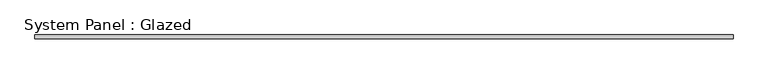
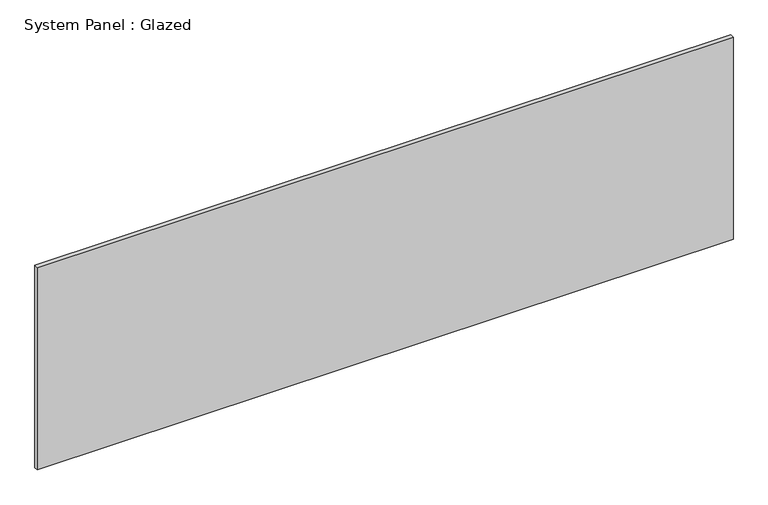
"""IFC4 building model written with IfcOpenShell, lengths in millimetres: plate geometry, System Panel : Glazed."""

from ifc_helpers import new_model, si_unit, origin, origin_with_axes, place, context, project, spatial, polyline, outline, extrude, source, transform, mapped, element, save


def system_panel_glazed_0e25fa2a(model_context):
    return source(origin(), model_context, "Body", "SweptSolid", [
        extrude(outline(polyline([(2374.9, 19.05), (-2374.9, 19.05), (-2374.9, 44.45), (2374.9, 44.45), (2374.9, 19.05)])), origin_with_axes(), (0.0, 0.0, 1.0), 1460.5),
    ])


if __name__ == "__main__":
    model = new_model("IFC4")
    model_context = context("Model", 3, world=origin())
    ifc_project = project(units=[si_unit("LENGTHUNIT", "METRE", prefix="MILLI")], contexts=[model_context])
    site = spatial("IfcSite", under=ifc_project)
    building = spatial("IfcBuilding", under=site)
    placement = place(None, origin())
    system_panel_glazed_shape = system_panel_glazed_0e25fa2a(model_context)
    element("IfcPlate", 1, ObjectType="System Panel : Glazed", at=placement, inside=building, context=model_context, shape_type="MappedRepresentation", body=[
        mapped(system_panel_glazed_shape, transform((0.0, 0.0, 0.0), x_axis=(1.0, 0.0, 0.0), y_axis=(0.0, 1.0, 0.0), z_axis=(0.0, 0.0, 1.0))),
    ])
    save(model, "model.ifc")

# Revit data of these elements
# Type "System Panel : Glazed"
#   Construction Type Id = "GSP4R"
#   Analytic Construction = "1/8 in Pilkington single glazing"
#   Visual Light Transmittance = 0.9
#   Solar Heat Gain Coefficient = 0.86
#   Heat Transfer Coefficient (U) = 1.18115 BTU/(h·ft²·°F)
# Element 1 (IfcPlate, "System Panel : Glazed")
#   Materials on its faces: "Glass"
# Materials
#   "Glass": class "Glass", colour RGB 0 128 192, transparency 0.75, Description = "Soda Lime Glass", Cost = 0
